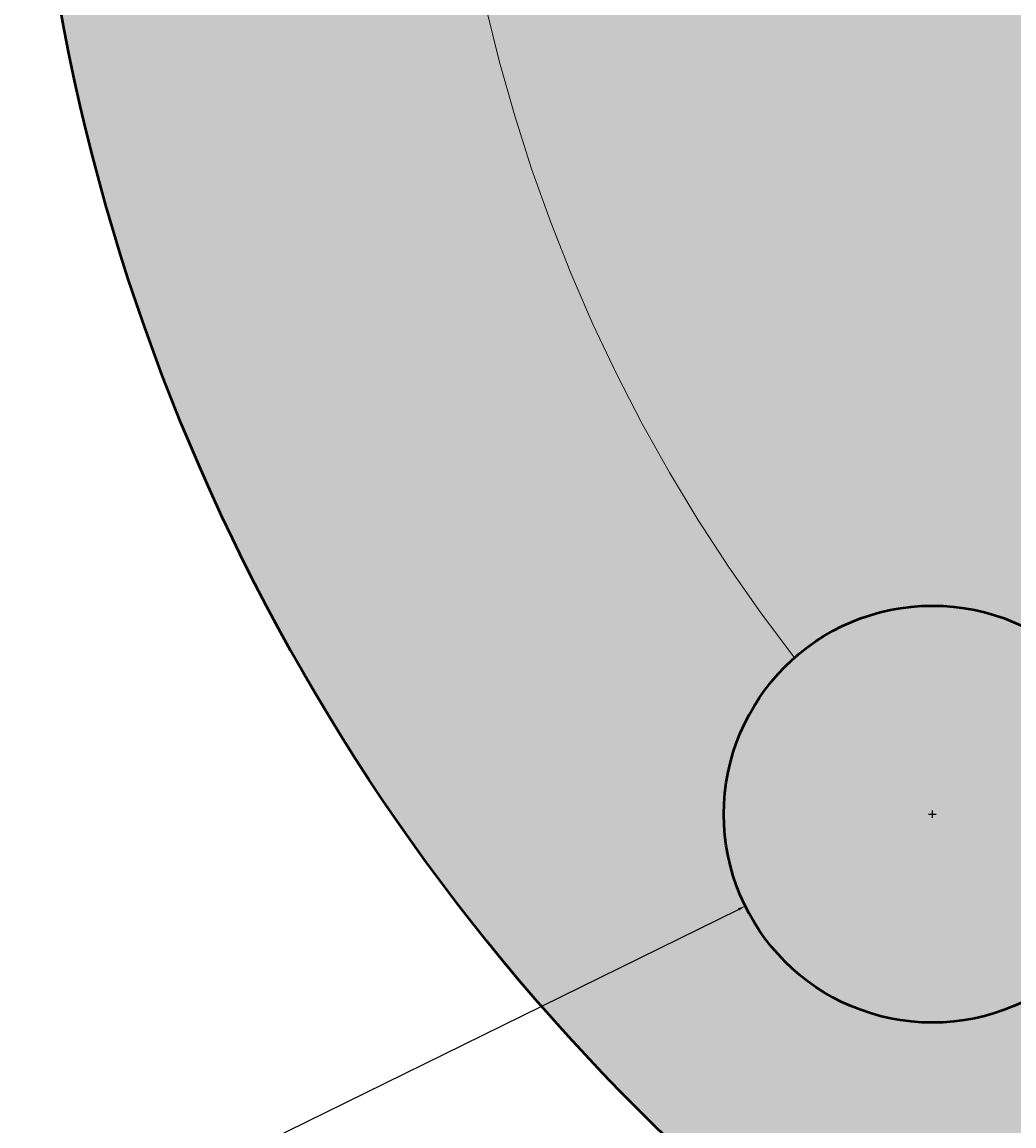
# Model space of a CAD drawing. Units: inches. Extents: x 139261 to 139415, y 52839 to 52963.
# Tile 2 of 20: x 139290 to 139314, y 52864 to 52891. Entities that reach past the tile are written whole.
import ezdxf

# ---------------------------------------------------------------- set-up
doc = ezdxf.new("R2010")
doc.units = ezdxf.units.IN
doc.header["$MEASUREMENT"] = 0
doc.linetypes.add('CENTER', pattern=[50.8, 31.75, -6.35, 6.35, -6.35])
for name, color, linetype, lineweight in [('M-CNTR', 4, 'CENTER', 18), ('M-DIMS', 2, 'Continuous', 25), ('M-HATC', 8, 'Continuous', 18), ('M-OUTL', 7, 'Continuous', 50)]:
    doc.layers.add(name, color=color, linetype=linetype, lineweight=lineweight)
doc.styles.get("Standard").update_dxf_attribs({"font": 'arial.ttf'})
doc.dimstyles.get("Standard").update_dxf_attribs({"dimtxt": 0.18, "dimasz": 0.18, "dimexe": 0.18, "dimexo": 0.0625, "dimgap": 0.09, "dimtad": 0, "dimtih": 1, "dimtoh": 1, "dimdec": 4, "dimzin": 0, "dimdsep": 46, "dimtxsty": 'Standard', "dimcen": 0.09, "dimadec": 0, "dimazin": 0, "dimtfac": 1, "dimtdec": 4, "dimtofl": 0, "dimtmove": 0, "dimatfit": 3, "dimfxl": 1, "dimtolj": 1, "dimtzin": 0, "dimarcsym": 0})

# ---------------------------------------------------------------- blocks, each defined once
blk = doc.blocks.new('*U1')
blk.add_circle((0, 0), 5)
blk = doc.blocks.new('*U2')
at = {"layer": 'M-OUTL', "color": 0, "linetype": 'ByBlock', "lineweight": -2, "transparency": 16777216, "rotation": 135}
blk.add_blockref('*U1', (139312.073, 52871.933), dxfattribs=at)
blk = doc.blocks.new('*D4')
at = {"layer": 'Defpoints', "color": 0, "transparency": 16777216}
for p in [(139373.053, 52923.26), (139307.661, 52877.175)]:
    blk.add_point(p, dxfattribs=at)
at = {"layer": 'M-DIMS', "color": 0, "lineweight": -2, "transparency": 16777216}
for p, q in [((139414.011, 52952.126), (139373.2, 52923.364)), ((139414.191, 52952.126), (139414.011, 52952.126)), ((139340.267, 52900.217), (139340.447, 52900.217)), ((139340.357, 52900.127), (139340.357, 52900.307))]:
    blk.add_line(p, q, dxfattribs=at)
blk.add_arc((139340.357, 52900.217), 40, 34.9168, 52.0771, dxfattribs=at)
at = {"layer": 'M-DIMS', "color": 0, "transparency": 16777216}
blk.add_solid([(139373.183, 52923.388), (139373.217, 52923.339), (139373.053, 52923.26)], dxfattribs=at)
at = {"layer": 'M-DIMS', "color": 0, "transparency": 16777216, "insert": (139414.822, 52952.126), "char_height": 0.18, "attachment_point": 5}
blk.add_mtext('\\A1;∅80.0000', dxfattribs=at)
blk = doc.blocks.new('*D7')
at = {"layer": 'Defpoints', "color": 0, "transparency": 16777216}
for p in [(139316.56, 52874.138), (139307.585, 52869.728)]:
    blk.add_point(p, dxfattribs=at)
at = {"layer": 'M-DIMS', "color": 0, "lineweight": -2, "transparency": 16777216}
for p, q in [((139312.073, 52871.843), (139312.073, 52872.023)), ((139311.983, 52871.933), (139312.163, 52871.933)), ((139282.904, 52857.598), (139307.424, 52869.649)), ((139282.724, 52857.598), (139282.904, 52857.598))]:
    blk.add_line(p, q, dxfattribs=at)
at = {"layer": 'M-DIMS', "color": 0, "transparency": 16777216}
blk.add_solid([(139307.41, 52869.675), (139307.437, 52869.622), (139307.585, 52869.728)], dxfattribs=at)
at = {"layer": 'M-DIMS', "color": 0, "transparency": 16777216, "insert": (139282.093, 52857.598), "char_height": 0.18, "attachment_point": 5}
blk.add_mtext('\\A1;∅10.0000', dxfattribs=at)
blk = doc.blocks.new('*D9')
at = {"layer": 'Defpoints', "color": 0, "transparency": 16777216}
for p in [(139302.054, 52932.357), (139378.659, 52868.078)]:
    blk.add_point(p, dxfattribs=at)
at = {"layer": 'M-DIMS', "color": 0, "lineweight": -2, "transparency": 16777216}
for p, q in [((139278.893, 52951.64), (139279.073, 52951.64)), ((139279.073, 52951.64), (139301.916, 52932.472)), ((139340.267, 52900.217), (139340.447, 52900.217)), ((139340.357, 52900.127), (139340.357, 52900.307))]:
    blk.add_line(p, q, dxfattribs=at)
at = {"layer": 'M-DIMS', "color": 0, "transparency": 16777216}
blk.add_solid([(139301.936, 52932.495), (139301.897, 52932.449), (139302.054, 52932.357)], dxfattribs=at)
at = {"layer": 'M-DIMS', "color": 0, "transparency": 16777216, "insert": (139278.506, 52951.64), "char_height": 0.18, "attachment_point": 5}
blk.add_mtext('\\A1;∅100', dxfattribs=at)

msp = doc.modelspace()

# ---------------------------------------------------------------- hatches: boundary and pattern name
at = {"layer": 'M-HATC'}
h = msp.add_hatch(color=256, dxfattribs=at)
h.dxf.hatch_style = 1
h.paths.add_polyline_path([(139290.35689, 52900.21749, 1), (139390.35689, 52900.21749, 1)])
h.paths.add_polyline_path([(139335.36666, 52939.90499, -0.01563646), (139335.35689, 52940.21749, -1), (139345.35689, 52940.21749, -0.01563646), (139345.34711, 52939.90499, -0.13461315), (139364.89157, 52931.80941, -0.691035), (139373.64116, 52928.50176, -0.21521822), (139371.94881, 52924.75216, -0.13461315), (139380.04439, 52905.20771, -0.43265224), (139385.35689, 52900.21749, -0.43265224), (139380.04439, 52895.22726, -0.13461315), (139371.94881, 52875.68281, -0.21521822), (139373.64116, 52871.93321, -0.691035), (139364.89157, 52868.62556, -0.13461315), (139345.34711, 52860.52999, -0.01563646), (139345.35689, 52860.21749, -1), (139335.35689, 52860.21749, -0.01563646), (139335.36666, 52860.52999, -0.13461315), (139315.82221, 52868.62556, -0.691035), (139307.07262, 52871.93321, -0.21521822), (139308.76496, 52875.68281, -0.13461315), (139300.66939, 52895.22726, -0.43265224), (139295.35689, 52900.21749, -0.43265224), (139300.66939, 52905.20771, -0.13461315), (139308.76496, 52924.75216, -0.21521822), (139307.07262, 52928.50176, -0.691035), (139315.82221, 52931.80941, -0.13461315)], flags=16)
h.paths.add_polyline_path([(139365.35689, 52900.21749, -1), (139315.35689, 52900.21749, -1)], flags=0)
h.paths.add_polyline_path([(139323.71474, 52911.30978), (139356.99903, 52911.30978, -0.3027197), (139356.99903, 52889.12519), (139323.71474, 52889.12519, -0.3027197)], flags=0)
h.paths.add_polyline_path([(139364.89157, 52931.80941, 0.13461315), (139345.34711, 52939.90499, -0.93933644), (139335.36666, 52939.90499, 0.13461315), (139315.82221, 52931.80941, -0.18270763), (139317.07262, 52928.50176, -0.64579494), (139308.76496, 52924.75216, 0.13461315), (139300.66939, 52905.20771, -0.39601219), (139305.35689, 52900.21749, -0.39601219), (139300.66939, 52895.22726, 0.13461315), (139308.76496, 52875.68281, -0.64579494), (139317.07262, 52871.93321, -0.18270763), (139315.82221, 52868.62556, 0.13461315), (139335.36666, 52860.52999, -0.93933644), (139345.34711, 52860.52999, 0.13461315), (139364.89157, 52868.62556, -0.18270763), (139363.64116, 52871.93321, -0.64579494), (139371.94881, 52875.68281, 0.13461315), (139380.04439, 52895.22726, -0.39601219), (139375.35689, 52900.21749, -0.39601219), (139380.04439, 52905.20771, 0.13461315), (139371.94881, 52924.75216, -0.64579494), (139363.64116, 52928.50176, -0.18270763)], flags=0)
h = msp.add_hatch(color=256, dxfattribs=at)
h.dxf.hatch_style = 1
h.set_gradient(color1=(205, 105, 40), tint=1)
h.paths.add_polyline_path([(139335.35689, 52940.21749, 1), (139345.35689, 52940.21749, 1)])
h.paths.add_polyline_path([(139307.07262, 52928.50176, 1), (139317.07262, 52928.50176, 1)])
h.paths.add_polyline_path([(139295.35689, 52900.21749, 1), (139305.35689, 52900.21749, 1)])
h.paths.add_polyline_path([(139307.07262, 52871.93321, 1), (139317.07262, 52871.93321, 1)])
h.paths.add_polyline_path([(139345.35689, 52860.21749, 1), (139335.35689, 52860.21749, 1)])
h.paths.add_polyline_path([(139363.64116, 52871.93321, 1), (139373.64116, 52871.93321, 1)])
h.paths.add_polyline_path([(139375.35689, 52900.21749, 1), (139385.35689, 52900.21749, 1)])
h.paths.add_polyline_path([(139363.64116, 52928.50176, 1), (139373.64116, 52928.50176, 1)])
h = msp.add_hatch(color=256, dxfattribs=at)
h.dxf.hatch_style = 1
h.paths.add_polyline_path([(139345.34711, 52939.90499, -0.93933644), (139335.36666, 52939.90499, 0.13461315), (139315.82221, 52931.80941, -0.18270763), (139317.07262, 52928.50176, -0.64579494), (139308.76496, 52924.75216, 0.13461315), (139300.66939, 52905.20771, -0.39601219), (139305.35689, 52900.21749, -0.39601219), (139300.66939, 52895.22726, 0.13461315), (139308.76496, 52875.68281, -0.64579494), (139317.07262, 52871.93321, -0.18270763), (139315.82221, 52868.62556, 0.13461315), (139335.36666, 52860.52999, -0.93933644), (139345.34711, 52860.52999, 0.13461315), (139364.89157, 52868.62556, -0.18270763), (139363.64116, 52871.93321, -0.64579494), (139371.94881, 52875.68281, 0.13461315), (139380.04439, 52895.22726, -0.39601219), (139375.35689, 52900.21749, -0.39601219), (139380.04439, 52905.20771, 0.13461315), (139371.94881, 52924.75216, -0.64579494), (139363.64116, 52928.50176, -0.18270763), (139364.89157, 52931.80941, 0.13461315)])
h.paths.add_polyline_path([(139365.35689, 52900.21749, -1), (139315.35689, 52900.21749, -1)], flags=16)
h.paths.add_polyline_path([(139356.99903, 52911.30978, -0.3027197), (139356.99903, 52889.12519), (139323.71474, 52889.12519, -0.3027197), (139323.71474, 52911.30978)], flags=0)

# ---------------------------------------------------------------- linework, layer by layer
at = {"layer": 'M-CNTR'}
msp.add_arc((139340.35689, 52900.21749), 40, 187.166643, 217.833357, dxfattribs=at)
at = {"layer": 'M-OUTL'}
msp.add_circle((139340.35689, 52900.21749), 50, dxfattribs=at)

# ---------------------------------------------------------------- block references
msp.add_blockref('*U2', (0, 0), dxfattribs=at)

# ---------------------------------------------------------------- dimensions: what is measured, and where the dimension line sits
at = {"layer": 'M-DIMS'}
for p1, p2, override, picture, middle in [((139307.66087, 52877.17469), (139373.0529, 52923.26028), {"dimclrd": 0, "dimclre": 0, "dimclrt": 0}, '*D4', (139414.82217, 52952.12585)), ((139378.65939, 52868.07845), (139302.05438, 52932.35652), {"dimdec": 0, "dimlfac": 1, "dimrnd": 0, "dimzin": 0, "dimdsep": 46, "dimlunit": 2}, '*D9', (139278.50641, 52951.63995)), ((139316.56001, 52874.1385), (139307.58522, 52869.72793), {"dimclrd": 0, "dimclre": 0, "dimclrt": 0}, '*D7', (139282.09259, 52857.59849))]:
    dim = msp.add_diameter_dim_2p(p1=p1, p2=p2, dimstyle='Standard', override=override, dxfattribs=at)
    dim.commit()
    dim.dimension.update_dxf_attribs({"geometry": picture, "text_midpoint": middle, "dimtype": 163})

doc.saveas('drawing.dxf')
